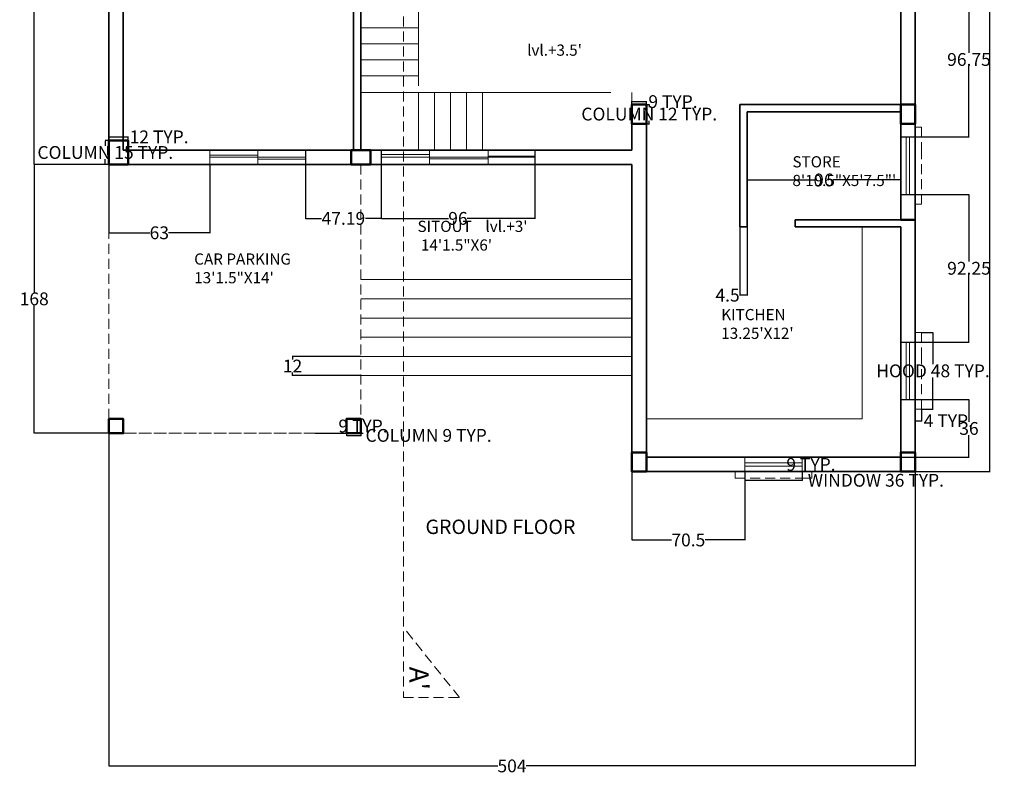
# Model space of a CAD drawing. Units: inches. Extents: x 683 to 1299, y -12 to 932.
# Tile 1 of 3: x 683 to 1299, y -12 to 460. Entities that reach past the tile are written whole.
import ezdxf

# ---------------------------------------------------------------- set-up
doc = ezdxf.new("R2010")
doc.units = ezdxf.units.IN
doc.header["$LTSCALE"] = 25
doc.header["$MEASUREMENT"] = 0
doc.linetypes.add('HIDDEN', pattern=[0.375, 0.25, -0.125])
for name, color, linetype, lineweight in [('A-ANNO-DIMS', 2, 'Continuous', 18), ('A-ANNO-SECT', 7, 'HIDDEN', 18), ('A-ANNO-SYMB', 6, 'Continuous', 18), ('A-ANNO-TEXT', 6, 'Continuous', 25), ('A-AREA-IDEN', 6, 'Continuous', 18), ('A-COLS', 1, 'Continuous', 50), ('A-FLOR', 7, 'Continuous', 25), ('A-FLOR-FIXT', 8, 'Continuous', 18), ('A-FLOR-STRS', 7, 'Continuous', 18), ('A-FLOR-STRS-HIDN', 5, 'HIDDEN', 18), ('A-GLAZ-OVHD', 7, 'HIDDEN', 13), ('A-ROOF-OVHD', 7, 'HIDDEN', 18), ('A-WALL', 7, 'Continuous', 35)]:
    doc.layers.add(name, color=color, linetype=linetype, lineweight=lineweight)
doc.layers.add('A-GLAZ', color=41, linetype='Continuous', lineweight=18, true_color=0xf4ee51)
doc.styles.get("Standard").update_dxf_attribs({"font": 'arial.ttf'})
doc.dimstyles.get("Standard").update_dxf_attribs({"dimtxt": 8, "dimasz": 0.18, "dimexe": 0.18, "dimexo": 0.0625, "dimgap": 0.09, "dimtad": 0, "dimtih": 1, "dimtoh": 1, "dimdec": 1, "dimzin": 0, "dimdsep": 46, "dimlunit": 3, "dimtxsty": 'Standard', "dimcen": 0.09, "dimadec": 0, "dimazin": 0, "dimtfac": 1, "dimtdec": 1, "dimtofl": 0, "dimtmove": 0, "dimatfit": 3, "dimfxl": 1, "dimtolj": 1, "dimtzin": 0, "dimarcsym": 0})

# ---------------------------------------------------------------- blocks, each defined once
blk = doc.blocks.new('WIN-SLIDER-60IN')
for p, q in [((60, 9), (0, 9)), ((0, 9), (0, 0)), ((30, 9), (30, 0)), ((60, 0), (60, 9)), ((0, 0), (60, 0)), ((30, 0), (60, 0))]:
    blk.add_line(p, q)
for points in [[(30, 4.5), (0, 4.5), (0, 5.76), (30, 5.76)], [(60, 3.24), (30, 3.24), (30, 4.5), (60, 4.5)]]:
    blk.add_lwpolyline(points, close=True)
blk = doc.blocks.new('WIN-36IN')
for p, q in [((36, 9), (0, 9)), ((0, 9), (0, 0)), ((36, 0), (36, 9)), ((0, 5.5), (36, 5.5)), ((0, 3.5), (36, 3.5)), ((0, 0), (36, 0))]:
    blk.add_line(p, q)
blk = doc.blocks.new('COLUMN-12X15IN')
blk.add_lwpolyline([(0, 0), (12, 0), (12, 15), (0, 15)], close=True)
blk = doc.blocks.new('COLUMN-12X9IN')
blk.add_lwpolyline([(0, 9), (0, 0), (12, 0), (12, 9)], close=True)
blk = doc.blocks.new('COLUMN-9X9IN')
blk.add_lwpolyline([(0, 0), (9, 0), (9, 9), (0, 9)], close=True)
blk = doc.blocks.new('WIN-HOOD-36IN')
for p, q in [((0, 48), (4, 48)), ((4, 48), (4, 33.44)), ((4, 0), (4, 33.44)), ((0, 0), (4, 0))]:
    blk.add_line(p, q)
blk = doc.blocks.new('*D14')
at = {"layer": 'A-ANNO-DIMS', "color": 0, "lineweight": -2, "ltscale": 25, "transparency": 16777216}
for p, q in [((1075.04, 407.1), (1076.95, 407.1)), ((1076.77, 406.92), (1076.77, 405.33)), ((1075.04, 395.1), (1076.95, 395.1)), ((1076.77, 395.28), (1076.77, 396.87))]:
    blk.add_line(p, q, dxfattribs=at)
at = {"layer": 'A-ANNO-DIMS', "color": 0, "ltscale": 25, "transparency": 16777216}
for points in [[(1076.74, 406.92), (1076.8, 406.92), (1076.77, 407.1)], [(1076.74, 395.28), (1076.8, 395.28), (1076.77, 395.1)]]:
    blk.add_solid(points, dxfattribs=at)
at = {"layer": 'Defpoints', "color": 0, "ltscale": 25, "transparency": 16777216}
for p in [(1074.97, 407.1), (1074.97, 395.1), (1076.77, 395.1)]:
    blk.add_point(p, dxfattribs=at)
at = {"layer": 'A-ANNO-DIMS', "color": 0, "ltscale": 25, "transparency": 16777216, "insert": (1076.77, 401.1), "char_height": 8, "attachment_point": 5}
blk.add_mtext('\\A1;COLUMN 12 TYP.', dxfattribs=at)
blk = doc.blocks.new('*D15')
at = {"layer": 'A-ANNO-DIMS', "color": 0, "lineweight": -2, "ltscale": 25, "transparency": 16777216}
for p, q in [((1065.97, 407.16), (1065.97, 409.08)), ((1066.15, 408.9), (1074.79, 408.9)), ((1074.97, 407.16), (1074.97, 409.08)), ((1074.97, 408.9), (1075.15, 408.9))]:
    blk.add_line(p, q, dxfattribs=at)
at = {"layer": 'A-ANNO-DIMS', "color": 0, "ltscale": 25, "transparency": 16777216}
for points in [[(1066.15, 408.93), (1066.15, 408.87), (1065.97, 408.9)], [(1074.79, 408.93), (1074.79, 408.87), (1074.97, 408.9)]]:
    blk.add_solid(points, dxfattribs=at)
at = {"layer": 'Defpoints', "color": 0, "ltscale": 25, "transparency": 16777216}
for p in [(1065.97, 407.1), (1074.97, 408.9), (1074.97, 407.1)]:
    blk.add_point(p, dxfattribs=at)
at = {"layer": 'A-ANNO-DIMS', "color": 0, "ltscale": 25, "transparency": 16777216, "insert": (1091.61, 408.9), "char_height": 8, "attachment_point": 5}
blk.add_mtext('\\A1;9 TYP.', dxfattribs=at)
blk = doc.blocks.new('*D16')
at = {"layer": 'A-ANNO-DIMS', "color": 0, "lineweight": -2, "ltscale": 25, "transparency": 16777216}
for p, q in [((1136.47, 177.54), (1136.47, 172.02)), ((1172.47, 177.54), (1172.47, 172.02)), ((1136.65, 172.2), (1172.29, 172.2)), ((1172.47, 172.2), (1172.65, 172.2))]:
    blk.add_line(p, q, dxfattribs=at)
at = {"layer": 'A-ANNO-DIMS', "color": 0, "ltscale": 25, "transparency": 16777216}
for points in [[(1136.65, 172.23), (1136.65, 172.17), (1136.47, 172.2)], [(1172.29, 172.23), (1172.29, 172.17), (1172.47, 172.2)]]:
    blk.add_solid(points, dxfattribs=at)
at = {"layer": 'Defpoints', "color": 0, "ltscale": 25, "transparency": 16777216}
for p in [(1136.47, 177.6), (1172.47, 177.6), (1172.47, 172.2)]:
    blk.add_point(p, dxfattribs=at)
at = {"layer": 'A-ANNO-DIMS', "color": 0, "ltscale": 25, "transparency": 16777216, "insert": (1218.45, 172.2), "char_height": 8, "attachment_point": 5}
blk.add_mtext('\\A1;WINDOW 36 TYP.', dxfattribs=at)
blk = doc.blocks.new('*D17')
at = {"layer": 'A-ANNO-DIMS', "color": 0, "lineweight": -2, "ltscale": 25, "transparency": 16777216}
for p, q in [((1172.54, 186.6), (1178.05, 186.6)), ((1177.87, 186.42), (1177.87, 186.27)), ((1172.54, 177.6), (1178.05, 177.6)), ((1177.87, 177.78), (1177.87, 177.92))]:
    blk.add_line(p, q, dxfattribs=at)
at = {"layer": 'A-ANNO-DIMS', "color": 0, "ltscale": 25, "transparency": 16777216}
for points in [[(1177.84, 186.42), (1177.9, 186.42), (1177.87, 186.6)], [(1177.84, 177.78), (1177.9, 177.78), (1177.87, 177.6)]]:
    blk.add_solid(points, dxfattribs=at)
at = {"layer": 'Defpoints', "color": 0, "ltscale": 25, "transparency": 16777216}
for p in [(1172.47, 186.6), (1177.87, 186.6), (1172.47, 177.6)]:
    blk.add_point(p, dxfattribs=at)
at = {"layer": 'A-ANNO-DIMS', "color": 0, "ltscale": 25, "transparency": 16777216, "insert": (1177.87, 182.1), "char_height": 8, "attachment_point": 5}
blk.add_mtext('\\A1;9 TYP.', dxfattribs=at)
blk = doc.blocks.new('*D20')
at = {"layer": 'A-ANNO-DIMS', "color": 0, "lineweight": -2, "ltscale": 25, "transparency": 16777216}
for p, q in [((738.91, 384.6), (736.54, 384.6)), ((736.72, 384.42), (736.72, 381.33)), ((738.91, 369.6), (736.54, 369.6)), ((736.72, 369.78), (736.72, 372.87))]:
    blk.add_line(p, q, dxfattribs=at)
at = {"layer": 'A-ANNO-DIMS', "color": 0, "ltscale": 25, "transparency": 16777216}
for points in [[(736.69, 384.42), (736.75, 384.42), (736.72, 384.6)], [(736.69, 369.78), (736.75, 369.78), (736.72, 369.6)]]:
    blk.add_solid(points, dxfattribs=at)
at = {"layer": 'Defpoints', "color": 0, "ltscale": 25, "transparency": 16777216}
for p in [(736.72, 384.6), (738.97, 384.6), (738.97, 369.6)]:
    blk.add_point(p, dxfattribs=at)
at = {"layer": 'A-ANNO-DIMS', "color": 0, "ltscale": 25, "transparency": 16777216, "insert": (736.72, 377.1), "char_height": 8, "attachment_point": 5}
blk.add_mtext('\\A1;COLUMN 15 TYP.', dxfattribs=at)
blk = doc.blocks.new('*D21')
at = {"layer": 'A-ANNO-DIMS', "color": 0, "lineweight": -2, "ltscale": 25, "transparency": 16777216}
for p, q in [((738.97, 384.66), (738.97, 387.03)), ((739.15, 386.85), (750.79, 386.85)), ((750.97, 384.66), (750.97, 387.03)), ((750.97, 386.85), (751.15, 386.85))]:
    blk.add_line(p, q, dxfattribs=at)
at = {"layer": 'A-ANNO-DIMS', "color": 0, "ltscale": 25, "transparency": 16777216}
for points in [[(739.15, 386.88), (739.15, 386.82), (738.97, 386.85)], [(750.79, 386.88), (750.79, 386.82), (750.97, 386.85)]]:
    blk.add_solid(points, dxfattribs=at)
at = {"layer": 'Defpoints', "color": 0, "ltscale": 25, "transparency": 16777216}
for p in [(738.97, 384.6), (750.97, 386.85), (750.97, 384.6)]:
    blk.add_point(p, dxfattribs=at)
at = {"layer": 'A-ANNO-DIMS', "color": 0, "ltscale": 25, "transparency": 16777216, "insert": (770.34, 386.85), "char_height": 8, "attachment_point": 5}
blk.add_mtext('\\A1;12 TYP.', dxfattribs=at)
blk = doc.blocks.new('*D22')
at = {"layer": 'A-ANNO-DIMS', "color": 0, "lineweight": -2, "ltscale": 25, "transparency": 16777216}
for p, q in [((887.47, 201.54), (887.47, 200.07)), ((887.65, 200.25), (896.29, 200.25)), ((896.47, 201.54), (896.47, 200.07)), ((896.47, 200.25), (896.65, 200.25))]:
    blk.add_line(p, q, dxfattribs=at)
at = {"layer": 'A-ANNO-DIMS', "color": 0, "ltscale": 25, "transparency": 16777216}
for points in [[(887.65, 200.28), (887.65, 200.22), (887.47, 200.25)], [(896.29, 200.28), (896.29, 200.22), (896.47, 200.25)]]:
    blk.add_solid(points, dxfattribs=at)
at = {"layer": 'Defpoints', "color": 0, "ltscale": 25, "transparency": 16777216}
for p in [(887.47, 201.6), (896.47, 201.6), (896.47, 200.25)]:
    blk.add_point(p, dxfattribs=at)
at = {"layer": 'A-ANNO-DIMS', "color": 0, "ltscale": 25, "transparency": 16777216, "insert": (938.83, 200.25), "char_height": 8, "attachment_point": 5}
blk.add_mtext('\\A1;COLUMN 9 TYP.', dxfattribs=at)
blk = doc.blocks.new('*D23')
at = {"layer": 'A-ANNO-DIMS', "color": 0, "lineweight": -2, "ltscale": 25, "transparency": 16777216}
for p, q in [((896.54, 210.6), (898, 210.6)), ((897.82, 210.42), (897.82, 210.27)), ((896.54, 201.6), (898, 201.6)), ((897.82, 201.78), (897.82, 201.92))]:
    blk.add_line(p, q, dxfattribs=at)
at = {"layer": 'A-ANNO-DIMS', "color": 0, "ltscale": 25, "transparency": 16777216}
for points in [[(897.79, 210.42), (897.85, 210.42), (897.82, 210.6)], [(897.79, 201.78), (897.85, 201.78), (897.82, 201.6)]]:
    blk.add_solid(points, dxfattribs=at)
at = {"layer": 'Defpoints', "color": 0, "ltscale": 25, "transparency": 16777216}
for p in [(896.47, 210.6), (897.82, 210.6), (896.47, 201.6)]:
    blk.add_point(p, dxfattribs=at)
at = {"layer": 'A-ANNO-DIMS', "color": 0, "ltscale": 25, "transparency": 16777216, "insert": (897.82, 206.1), "char_height": 8, "attachment_point": 5}
blk.add_mtext('\\A1;9 TYP.', dxfattribs=at)
blk = doc.blocks.new('*D28')
at = {"layer": 'A-ANNO-DIMS', "color": 0, "lineweight": -2, "ltscale": 25, "transparency": 16777216}
for p, q in [((1247.04, 264.6), (1254.35, 264.6)), ((1254.17, 264.42), (1254.17, 244.83)), ((1254.17, 216.78), (1254.17, 236.37)), ((1247.04, 216.6), (1254.35, 216.6))]:
    blk.add_line(p, q, dxfattribs=at)
at = {"layer": 'A-ANNO-DIMS', "color": 0, "ltscale": 25, "transparency": 16777216}
for points in [[(1254.14, 264.42), (1254.2, 264.42), (1254.17, 264.6)], [(1254.14, 216.78), (1254.2, 216.78), (1254.17, 216.6)]]:
    blk.add_solid(points, dxfattribs=at)
at = {"layer": 'Defpoints', "color": 0, "ltscale": 25, "transparency": 16777216}
for p in [(1246.97, 264.6), (1254.17, 264.6), (1246.97, 216.6)]:
    blk.add_point(p, dxfattribs=at)
at = {"layer": 'A-ANNO-DIMS', "color": 0, "ltscale": 25, "transparency": 16777216, "insert": (1254.17, 240.6), "char_height": 8, "attachment_point": 5}
blk.add_mtext('\\A1;HOOD 48 TYP.', dxfattribs=at)
blk = doc.blocks.new('*D29')
at = {"layer": 'A-ANNO-DIMS', "color": 0, "lineweight": -2, "ltscale": 25, "transparency": 16777216}
for p, q in [((1242.97, 216.54), (1242.97, 209.22)), ((1246.97, 216.54), (1246.97, 209.22)), ((1243.15, 209.4), (1246.79, 209.4)), ((1246.97, 209.4), (1247.15, 209.4))]:
    blk.add_line(p, q, dxfattribs=at)
at = {"layer": 'A-ANNO-DIMS', "color": 0, "ltscale": 25, "transparency": 16777216}
for points in [[(1243.15, 209.43), (1243.15, 209.37), (1242.97, 209.4)], [(1246.79, 209.43), (1246.79, 209.37), (1246.97, 209.4)]]:
    blk.add_solid(points, dxfattribs=at)
at = {"layer": 'Defpoints', "color": 0, "ltscale": 25, "transparency": 16777216}
for p in [(1242.97, 216.6), (1246.97, 216.6), (1246.97, 209.4)]:
    blk.add_point(p, dxfattribs=at)
at = {"layer": 'A-ANNO-DIMS', "color": 0, "ltscale": 25, "transparency": 16777216, "insert": (1263.77, 209.4), "char_height": 8, "attachment_point": 5}
blk.add_mtext('\\A1;4 TYP.', dxfattribs=at)
blk = doc.blocks.new('*D32')
at = {"layer": 'A-ANNO-DIMS', "color": 0, "lineweight": -2, "ltscale": 25, "transparency": 16777216}
for p, q in [((738.97, 201.54), (738.97, -6.53)), ((1242.97, 177.54), (1242.97, -6.53)), ((739.15, -6.35), (982.06, -6.35)), ((1242.79, -6.35), (999.88, -6.35))]:
    blk.add_line(p, q, dxfattribs=at)
at = {"layer": 'A-ANNO-DIMS', "color": 0, "ltscale": 25, "transparency": 16777216}
for points in [[(739.15, -6.32), (739.15, -6.38), (738.97, -6.35)], [(1242.79, -6.32), (1242.79, -6.38), (1242.97, -6.35)]]:
    blk.add_solid(points, dxfattribs=at)
at = {"layer": 'Defpoints', "color": 0, "ltscale": 25, "transparency": 16777216}
for p in [(738.97, 201.6), (1242.97, 177.6), (1242.97, -6.35)]:
    blk.add_point(p, dxfattribs=at)
at = {"layer": 'A-ANNO-DIMS', "color": 0, "ltscale": 25, "transparency": 16777216, "insert": (990.97, -6.35), "char_height": 8, "attachment_point": 5}
blk.add_mtext('\\A1;504', dxfattribs=at)
blk = doc.blocks.new('*D33')
at = {"layer": 'A-ANNO-DIMS', "color": 0, "lineweight": -2, "ltscale": 25, "transparency": 16777216}
for p, q in [((1243.04, 825.6), (1289.85, 825.6)), ((1289.67, 825.42), (1289.67, 505.77)), ((1289.67, 177.78), (1289.67, 497.42)), ((1243.04, 177.6), (1289.85, 177.6))]:
    blk.add_line(p, q, dxfattribs=at)
at = {"layer": 'A-ANNO-DIMS', "color": 0, "ltscale": 25, "transparency": 16777216}
for points in [[(1289.64, 825.42), (1289.7, 825.42), (1289.67, 825.6)], [(1289.64, 177.78), (1289.7, 177.78), (1289.67, 177.6)]]:
    blk.add_solid(points, dxfattribs=at)
at = {"layer": 'Defpoints', "color": 0, "ltscale": 25, "transparency": 16777216}
for p in [(1242.97, 825.6), (1289.67, 825.6), (1242.97, 177.6)]:
    blk.add_point(p, dxfattribs=at)
at = {"layer": 'A-ANNO-DIMS', "color": 0, "ltscale": 25, "transparency": 16777216, "insert": (1289.67, 501.6), "char_height": 8, "attachment_point": 5}
blk.add_mtext('\\A1;648', dxfattribs=at)
blk = doc.blocks.new('*D40')
at = {"layer": 'A-ANNO-DIMS', "color": 0, "lineweight": -2, "ltscale": 25, "transparency": 16777216}
for p, q in [((738.91, 369.6), (692.09, 369.6)), ((692.27, 369.42), (692.27, 289.77)), ((692.27, 201.78), (692.27, 281.42)), ((738.91, 201.6), (692.09, 201.6))]:
    blk.add_line(p, q, dxfattribs=at)
at = {"layer": 'A-ANNO-DIMS', "color": 0, "ltscale": 25, "transparency": 16777216}
for points in [[(692.24, 369.42), (692.3, 369.42), (692.27, 369.6)], [(692.24, 201.78), (692.3, 201.78), (692.27, 201.6)]]:
    blk.add_solid(points, dxfattribs=at)
at = {"layer": 'Defpoints', "color": 0, "ltscale": 25, "transparency": 16777216}
for p in [(692.27, 369.6), (738.97, 369.6), (738.97, 201.6)]:
    blk.add_point(p, dxfattribs=at)
at = {"layer": 'A-ANNO-DIMS', "color": 0, "ltscale": 25, "transparency": 16777216, "insert": (692.27, 285.6), "char_height": 8, "attachment_point": 5}
blk.add_mtext('\\A1;168', dxfattribs=at)
blk = doc.blocks.new('*D41')
at = {"layer": 'A-ANNO-DIMS', "color": 0, "lineweight": -2, "ltscale": 25, "transparency": 16777216}
for p, q in [((738.91, 570.6), (692.09, 570.6)), ((692.27, 570.42), (692.27, 474.27)), ((692.27, 369.78), (692.27, 465.92)), ((738.91, 369.6), (692.09, 369.6))]:
    blk.add_line(p, q, dxfattribs=at)
at = {"layer": 'A-ANNO-DIMS', "color": 0, "ltscale": 25, "transparency": 16777216}
for points in [[(692.24, 570.42), (692.3, 570.42), (692.27, 570.6)], [(692.24, 369.78), (692.3, 369.78), (692.27, 369.6)]]:
    blk.add_solid(points, dxfattribs=at)
at = {"layer": 'Defpoints', "color": 0, "ltscale": 25, "transparency": 16777216}
for p in [(692.27, 570.6), (738.97, 570.6), (738.97, 369.6)]:
    blk.add_point(p, dxfattribs=at)
at = {"layer": 'A-ANNO-DIMS', "color": 0, "ltscale": 25, "transparency": 16777216, "insert": (692.27, 470.1), "char_height": 8, "attachment_point": 5}
blk.add_mtext('\\A1;201', dxfattribs=at)
blk = doc.blocks.new('*D47')
at = {"layer": 'A-ANNO-DIMS', "color": 0, "lineweight": -2, "ltscale": 25, "transparency": 16777216}
for p, q in [((1234.04, 483.6), (1276.85, 483.6)), ((1276.67, 483.42), (1276.67, 439.4)), ((1276.67, 387.03), (1276.67, 431.05)), ((1234.04, 386.85), (1276.85, 386.85))]:
    blk.add_line(p, q, dxfattribs=at)
at = {"layer": 'A-ANNO-DIMS', "color": 0, "ltscale": 25, "transparency": 16777216}
for points in [[(1276.64, 483.42), (1276.7, 483.42), (1276.67, 483.6)], [(1276.64, 387.03), (1276.7, 387.03), (1276.67, 386.85)]]:
    blk.add_solid(points, dxfattribs=at)
at = {"layer": 'Defpoints', "color": 0, "ltscale": 25, "transparency": 16777216}
for p in [(1233.97, 483.6), (1233.97, 386.85), (1276.67, 386.85)]:
    blk.add_point(p, dxfattribs=at)
at = {"layer": 'A-ANNO-DIMS', "color": 0, "ltscale": 25, "transparency": 16777216, "insert": (1276.67, 435.22), "char_height": 8, "attachment_point": 5}
blk.add_mtext('\\A1;96.75', dxfattribs=at)
blk = doc.blocks.new('*D48')
at = {"layer": 'A-ANNO-DIMS', "color": 0, "lineweight": -2, "ltscale": 25, "transparency": 16777216}
for p, q in [((1234.04, 350.85), (1276.85, 350.85)), ((1276.67, 350.67), (1276.67, 308.9)), ((1276.67, 258.78), (1276.67, 300.55)), ((1234.04, 258.6), (1276.85, 258.6))]:
    blk.add_line(p, q, dxfattribs=at)
at = {"layer": 'A-ANNO-DIMS', "color": 0, "ltscale": 25, "transparency": 16777216}
for points in [[(1276.64, 350.67), (1276.7, 350.67), (1276.67, 350.85)], [(1276.64, 258.78), (1276.7, 258.78), (1276.67, 258.6)]]:
    blk.add_solid(points, dxfattribs=at)
at = {"layer": 'Defpoints', "color": 0, "ltscale": 25, "transparency": 16777216}
for p in [(1233.97, 350.85), (1233.97, 258.6), (1276.67, 258.6)]:
    blk.add_point(p, dxfattribs=at)
at = {"layer": 'A-ANNO-DIMS', "color": 0, "ltscale": 25, "transparency": 16777216, "insert": (1276.67, 304.72), "char_height": 8, "attachment_point": 5}
blk.add_mtext('\\A1;92.25', dxfattribs=at)
blk = doc.blocks.new('*D49')
at = {"layer": 'A-ANNO-DIMS', "color": 0, "lineweight": -2, "ltscale": 25, "transparency": 16777216}
for p, q in [((1234.04, 222.6), (1276.85, 222.6)), ((1276.67, 222.42), (1276.67, 208.78)), ((1276.67, 186.78), (1276.67, 200.42)), ((1234.04, 186.6), (1276.85, 186.6))]:
    blk.add_line(p, q, dxfattribs=at)
at = {"layer": 'A-ANNO-DIMS', "color": 0, "ltscale": 25, "transparency": 16777216}
for points in [[(1276.64, 222.42), (1276.7, 222.42), (1276.67, 222.6)], [(1276.64, 186.78), (1276.7, 186.78), (1276.67, 186.6)]]:
    blk.add_solid(points, dxfattribs=at)
at = {"layer": 'Defpoints', "color": 0, "ltscale": 25, "transparency": 16777216}
for p in [(1233.97, 222.6), (1233.97, 186.6), (1276.67, 186.6)]:
    blk.add_point(p, dxfattribs=at)
at = {"layer": 'A-ANNO-DIMS', "color": 0, "ltscale": 25, "transparency": 16777216, "insert": (1276.67, 204.6), "char_height": 8, "attachment_point": 5}
blk.add_mtext('\\A1;36', dxfattribs=at)
blk = doc.blocks.new('*D52')
at = {"layer": 'A-ANNO-DIMS', "color": 0, "lineweight": -2, "ltscale": 25, "transparency": 16777216}
for p, q in [((896.41, 249.6), (853.59, 249.6)), ((853.77, 249.42), (853.77, 247.71)), ((896.41, 237.6), (853.59, 237.6)), ((853.77, 237.78), (853.77, 239.49))]:
    blk.add_line(p, q, dxfattribs=at)
at = {"layer": 'A-ANNO-DIMS', "color": 0, "ltscale": 25, "transparency": 16777216}
for points in [[(853.74, 249.42), (853.8, 249.42), (853.77, 249.6)], [(853.74, 237.78), (853.8, 237.78), (853.77, 237.6)]]:
    blk.add_solid(points, dxfattribs=at)
at = {"layer": 'Defpoints', "color": 0, "ltscale": 25, "transparency": 16777216}
for p in [(853.77, 249.6), (896.47, 249.6), (896.47, 237.6)]:
    blk.add_point(p, dxfattribs=at)
at = {"layer": 'A-ANNO-DIMS', "color": 0, "ltscale": 25, "transparency": 16777216, "insert": (853.77, 243.6), "char_height": 8, "attachment_point": 5}
blk.add_mtext('\\A1;12', dxfattribs=at)
blk = doc.blocks.new('*D55')
at = {"layer": 'A-ANNO-DIMS', "color": 0, "lineweight": -2, "ltscale": 25, "transparency": 16777216}
for p, q in [((738.97, 369.54), (738.97, 326.72)), ((801.97, 369.54), (801.97, 326.72)), ((739.15, 326.9), (764.63, 326.9)), ((801.79, 326.9), (776.31, 326.9))]:
    blk.add_line(p, q, dxfattribs=at)
at = {"layer": 'A-ANNO-DIMS', "color": 0, "ltscale": 25, "transparency": 16777216}
for points in [[(739.15, 326.93), (739.15, 326.87), (738.97, 326.9)], [(801.79, 326.93), (801.79, 326.87), (801.97, 326.9)]]:
    blk.add_solid(points, dxfattribs=at)
at = {"layer": 'Defpoints', "color": 0, "ltscale": 25, "transparency": 16777216}
for p in [(738.97, 369.6), (801.97, 369.6), (738.97, 326.9)]:
    blk.add_point(p, dxfattribs=at)
at = {"layer": 'A-ANNO-DIMS', "color": 0, "ltscale": 25, "transparency": 16777216, "insert": (770.47, 326.9), "char_height": 8, "attachment_point": 5}
blk.add_mtext('\\A1;63', dxfattribs=at)
blk = doc.blocks.new('*D56')
at = {"layer": 'A-ANNO-DIMS', "color": 0, "lineweight": -2, "ltscale": 25, "transparency": 16777216}
for p, q in [((861.97, 378.54), (861.97, 335.72)), ((909.17, 378.54), (909.17, 335.72)), ((862.15, 335.9), (871.81, 335.9)), ((908.99, 335.9), (899.33, 335.9))]:
    blk.add_line(p, q, dxfattribs=at)
at = {"layer": 'A-ANNO-DIMS', "color": 0, "ltscale": 25, "transparency": 16777216}
for points in [[(862.15, 335.93), (862.15, 335.87), (861.97, 335.9)], [(908.99, 335.93), (908.99, 335.87), (909.17, 335.9)]]:
    blk.add_solid(points, dxfattribs=at)
at = {"layer": 'Defpoints', "color": 0, "ltscale": 25, "transparency": 16777216}
for p in [(861.97, 378.6), (909.17, 378.6), (861.97, 335.9)]:
    blk.add_point(p, dxfattribs=at)
at = {"layer": 'A-ANNO-DIMS', "color": 0, "ltscale": 25, "transparency": 16777216, "insert": (885.57, 335.9), "char_height": 8, "attachment_point": 5}
blk.add_mtext('\\A1;47.19', dxfattribs=at)
blk = doc.blocks.new('*D57')
at = {"layer": 'A-ANNO-DIMS', "color": 0, "lineweight": -2, "ltscale": 25, "transparency": 16777216}
for p, q in [((909.17, 378.54), (909.17, 335.72)), ((1005.17, 378.54), (1005.17, 335.72)), ((909.35, 335.9), (951.35, 335.9)), ((1004.99, 335.9), (962.98, 335.9))]:
    blk.add_line(p, q, dxfattribs=at)
at = {"layer": 'A-ANNO-DIMS', "color": 0, "ltscale": 25, "transparency": 16777216}
for points in [[(909.35, 335.93), (909.35, 335.87), (909.17, 335.9)], [(1004.99, 335.93), (1004.99, 335.87), (1005.17, 335.9)]]:
    blk.add_solid(points, dxfattribs=at)
at = {"layer": 'Defpoints', "color": 0, "ltscale": 25, "transparency": 16777216}
for p in [(909.17, 378.6), (1005.17, 378.6), (909.17, 335.9)]:
    blk.add_point(p, dxfattribs=at)
at = {"layer": 'A-ANNO-DIMS', "color": 0, "ltscale": 25, "transparency": 16777216, "insert": (957.17, 335.9), "char_height": 8, "attachment_point": 5}
blk.add_mtext('\\A1;96', dxfattribs=at)
blk = doc.blocks.new('*D58')
at = {"layer": 'A-ANNO-DIMS', "color": 0, "lineweight": -2, "ltscale": 25, "transparency": 16777216}
for p, q in [((1065.97, 177.54), (1065.97, 134.72)), ((1136.47, 177.54), (1136.47, 134.72)), ((1066.15, 134.9), (1090.75, 134.9)), ((1136.29, 134.9), (1111.7, 134.9))]:
    blk.add_line(p, q, dxfattribs=at)
at = {"layer": 'A-ANNO-DIMS', "color": 0, "ltscale": 25, "transparency": 16777216}
for points in [[(1066.15, 134.93), (1066.15, 134.87), (1065.97, 134.9)], [(1136.29, 134.93), (1136.29, 134.87), (1136.47, 134.9)]]:
    blk.add_solid(points, dxfattribs=at)
at = {"layer": 'Defpoints', "color": 0, "ltscale": 25, "transparency": 16777216}
for p in [(1065.97, 177.6), (1136.47, 177.6), (1065.97, 134.9)]:
    blk.add_point(p, dxfattribs=at)
at = {"layer": 'A-ANNO-DIMS', "color": 0, "ltscale": 25, "transparency": 16777216, "insert": (1101.22, 134.9), "char_height": 8, "attachment_point": 5}
blk.add_mtext('\\A1;70.5', dxfattribs=at)
blk = doc.blocks.new('*D59')
at = {"layer": 'A-ANNO-DIMS', "color": 0, "lineweight": -2, "ltscale": 25, "transparency": 16777216}
for p, q in [((1137.97, 402.54), (1137.97, 359.72)), ((1233.97, 402.54), (1233.97, 359.72)), ((1138.15, 359.9), (1180.16, 359.9)), ((1233.79, 359.9), (1191.79, 359.9))]:
    blk.add_line(p, q, dxfattribs=at)
at = {"layer": 'A-ANNO-DIMS', "color": 0, "ltscale": 25, "transparency": 16777216}
for points in [[(1138.15, 359.93), (1138.15, 359.87), (1137.97, 359.9)], [(1233.79, 359.93), (1233.79, 359.87), (1233.97, 359.9)]]:
    blk.add_solid(points, dxfattribs=at)
at = {"layer": 'Defpoints', "color": 0, "ltscale": 25, "transparency": 16777216}
for p in [(1137.97, 402.6), (1233.97, 402.6), (1137.97, 359.9)]:
    blk.add_point(p, dxfattribs=at)
at = {"layer": 'A-ANNO-DIMS', "color": 0, "ltscale": 25, "transparency": 16777216, "insert": (1185.97, 359.9), "char_height": 8, "attachment_point": 5}
blk.add_mtext('\\A1;96', dxfattribs=at)
blk = doc.blocks.new('*D60')
at = {"layer": 'A-ANNO-DIMS', "color": 0, "lineweight": -2, "ltscale": 25, "transparency": 16777216}
for p, q in [((1133.47, 330.54), (1133.47, 287.72)), ((1137.97, 330.54), (1137.97, 287.72)), ((1133.47, 287.9), (1133.29, 287.9)), ((1137.79, 287.9), (1133.65, 287.9))]:
    blk.add_line(p, q, dxfattribs=at)
at = {"layer": 'A-ANNO-DIMS', "color": 0, "ltscale": 25, "transparency": 16777216}
for points in [[(1133.65, 287.93), (1133.65, 287.87), (1133.47, 287.9)], [(1137.79, 287.93), (1137.79, 287.87), (1137.97, 287.9)]]:
    blk.add_solid(points, dxfattribs=at)
at = {"layer": 'Defpoints', "color": 0, "ltscale": 25, "transparency": 16777216}
for p in [(1133.47, 330.6), (1137.97, 330.6), (1133.47, 287.9)]:
    blk.add_point(p, dxfattribs=at)
at = {"layer": 'A-ANNO-DIMS', "color": 0, "ltscale": 25, "transparency": 16777216, "insert": (1125.73, 287.9), "char_height": 8, "attachment_point": 5}
blk.add_mtext('\\A1;4.5', dxfattribs=at)

msp = doc.modelspace()

# ---------------------------------------------------------------- linework, layer by layer
at = {"layer": 'A-ANNO-SECT'}
for p, q in [((923.068, 883.972), (923.068, 36.355)), ((958.231, 36.355), (923.068, 80.211)), ((923.068, 36.355), (958.231, 36.355))]:
    msp.add_line(p, q, dxfattribs=at)
at = {"layer": 'A-COLS'}
for p, q in [((1065.973, 407.099), (1074.973, 407.099)), ((1233.973, 407.099), (1242.973, 407.099)), ((1233.973, 335.099), (1242.973, 335.099)), ((738.973, 210.599), (738.973, 201.599)), ((1065.973, 189.599), (1074.973, 189.599)), ((1233.973, 189.599), (1242.973, 189.599))]:
    msp.add_line(p, q, dxfattribs=at)
at = {"layer": 'A-FLOR'}
for p, q in [((896.473, 369.599), (1065.973, 369.599)), ((867.973, 201.599), (896.473, 201.599))]:
    msp.add_line(p, q, dxfattribs=at)
at = {"layer": 'A-FLOR-FIXT'}
for p in [(1209.973, 330.599), (1074.973, 210.599)]:
    msp.add_line(p, (1209.973, 210.599), dxfattribs=at)
at = {"layer": 'A-FLOR-STRS'}
for p, q in [((896.473, 297.599), (1065.973, 297.599)), ((896.473, 285.599), (1065.973, 285.599)), ((896.473, 273.599), (1065.973, 273.599)), ((896.473, 261.599), (1065.973, 261.599)), ((896.473, 249.599), (1065.973, 249.599)), ((896.473, 237.599), (1065.973, 237.599))]:
    msp.add_line(p, q, dxfattribs=at)
at = {"layer": 'A-FLOR-STRS-HIDN', "ltscale": 25}
for p, q in [((932.473, 575.099), (932.473, 378.599)), ((932.473, 455.099), (896.473, 455.099)), ((932.473, 445.099), (896.473, 445.099)), ((932.473, 435.099), (896.473, 435.099)), ((932.473, 425.099), (896.473, 425.099)), ((896.473, 414.599), (1065.973, 414.599)), ((932.473, 414.618), (898.973, 414.618)), ((932.473, 414.618), (898.973, 414.618)), ((932.473, 414.618), (898.973, 414.618)), ((932.473, 414.599), (932.473, 378.599)), ((942.473, 414.599), (942.473, 378.599)), ((952.473, 414.599), (952.473, 378.599)), ((962.473, 414.599), (962.473, 378.599)), ((972.473, 414.599), (972.473, 378.599)), ((1065.973, 407.099), (1065.973, 414.599))]:
    msp.add_line(p, q, dxfattribs=at)
at = {"layer": 'A-GLAZ'}
for p, q in [((1242.973, 386.849), (1242.973, 392.849)), ((1233.973, 368.849), (1233.973, 386.849)), ((1242.973, 350.849), (1242.973, 386.849)), ((801.973, 369.599), (801.973, 378.599)), ((801.973, 378.599), (837.973, 378.599)), ((819.973, 378.599), (837.973, 378.599)), ((1005.166, 378.599), (909.166, 378.599)), ((909.166, 378.599), (909.166, 369.599)), ((939.348, 369.599), (939.348, 378.599)), ((975.997, 369.599), (975.997, 378.599)), ((1005.166, 369.599), (1005.166, 378.599)), ((837.973, 369.599), (801.973, 369.599)), ((909.166, 369.599), (1005.166, 369.599)), ((957.166, 369.599), (1005.166, 369.599)), ((1242.973, 350.849), (1242.973, 344.849)), ((1242.973, 258.599), (1242.973, 264.599)), ((1242.973, 222.599), (1242.973, 216.599)), ((1136.473, 177.599), (1130.473, 177.599)), ((1154.473, 177.599), (1172.473, 177.599)), ((1172.473, 177.599), (1178.473, 177.599))]:
    msp.add_line(p, q, dxfattribs=at)
for points in [[(939.348, 374.099), (909.166, 374.099), (909.166, 375.825), (939.348, 375.825)], [(939.348, 374.099), (975.997, 374.099), (975.997, 373.034), (939.348, 373.034)], [(975.997, 374.099), (1005.166, 374.099), (1005.166, 374.891), (975.997, 374.891)]]:
    msp.add_lwpolyline(points, close=True, dxfattribs=at)
at = {"layer": 'A-GLAZ-OVHD'}
for p, q in [((1130.473, 177.599), (1130.473, 173.599)), ((1130.473, 173.599), (1174.082, 173.599)), ((1178.473, 173.599), (1174.082, 173.599)), ((1178.473, 177.599), (1178.473, 173.599))]:
    msp.add_line(p, q, dxfattribs=at)
at = {"layer": 'A-ROOF-OVHD'}
for p, q in [((738.973, 210.599), (738.973, 369.599)), ((896.473, 369.599), (896.473, 201.599)), ((896.473, 369.599), (896.473, 210.599)), ((738.973, 201.599), (867.973, 201.599)), ((887.473, 201.599), (747.973, 201.599))]:
    msp.add_line(p, q, dxfattribs=at)
at = {"layer": 'A-WALL'}
for p, q in [((738.973, 825.599), (738.973, 369.599)), ((1242.973, 729.599), (1242.973, 177.599)), ((1233.973, 620.099), (1233.973, 407.099)), ((896.473, 575.099), (896.473, 378.599)), ((747.973, 570.599), (747.973, 378.599)), ((891.973, 570.599), (891.973, 378.599)), ((1065.973, 407.099), (1065.973, 378.599)), ((1074.973, 407.099), (1074.973, 251.778)), ((1133.473, 407.099), (1133.473, 330.599)), ((1133.473, 407.099), (1233.973, 407.099)), ((1137.973, 402.599), (1137.973, 335.099)), ((1137.973, 402.599), (1233.973, 402.599)), ((1233.973, 402.599), (1233.973, 335.099)), ((747.973, 378.599), (891.973, 378.599)), ((896.473, 378.599), (1065.973, 378.599)), ((738.973, 369.599), (1065.973, 369.599)), ((1065.973, 369.599), (1065.973, 177.599)), ((1137.973, 335.099), (1137.973, 330.599)), ((1167.973, 335.099), (1233.973, 335.099)), ((1167.973, 335.099), (1167.973, 330.599)), ((1074.973, 330.599), (1074.973, 186.599)), ((1133.473, 330.599), (1137.973, 330.599)), ((1167.973, 330.599), (1233.973, 330.599)), ((1233.973, 330.599), (1233.973, 186.599)), ((1074.973, 186.599), (1233.973, 186.599)), ((1065.973, 177.599), (1242.973, 177.599))]:
    msp.add_line(p, q, dxfattribs=at)

# ---------------------------------------------------------------- block references
at = {"layer": 'A-COLS'}
for p, rotation in [((1065.973, 407.099), 269.9999999999999), ((1233.973, 407.099), 269.9999999999999), ((1065.973, 189.599), 270), ((1233.973, 189.599), 270)]:
    msp.add_blockref('COLUMN-12X9IN', p, dxfattribs=dict(at, rotation=rotation))
for name, p in [('COLUMN-12X15IN', (738.973, 369.599)), ('COLUMN-12X9IN', (890.473, 369.599)), ('COLUMN-9X9IN', (738.973, 201.599)), ('COLUMN-9X9IN', (887.473, 201.599))]:
    msp.add_blockref(name, p, dxfattribs=at)
at = {"layer": 'A-GLAZ'}
for p, rotation in [((1242.973, 350.849), 89.99999999999962), ((1242.973, 222.599), 89.99999999999959)]:
    msp.add_blockref('WIN-36IN', p, dxfattribs=dict(at, rotation=rotation))
for name, p in [('WIN-SLIDER-60IN', (801.973, 369.599)), ('WIN-36IN', (1136.473, 177.599))]:
    msp.add_blockref(name, p, dxfattribs=at)
at = {"layer": 'A-GLAZ-OVHD'}
for p in [(1242.973, 344.849), (1242.973, 216.599)]:
    msp.add_blockref('WIN-HOOD-36IN', p, dxfattribs=at)

# ---------------------------------------------------------------- texts
at = {"layer": 'A-ANNO-SECT', "ltscale": 25, "insert": (938.851, 55.648), "char_height": 12, "attachment_point": 1, "rotation": 270}
msp.add_mtext_dynamic_manual_height_columns("A'", width=16.69857, gutter_width=1, heights=[0], dxfattribs=at)
at = {"layer": 'A-ANNO-SYMB', "ltscale": 25, "insert": (993.426, 444.574), "char_height": 7, "attachment_point": 1}
msp.add_mtext_dynamic_manual_height_columns("\\pxi-3,l4,t4;lvl.+3.5'", width=117.16603, gutter_width=1, heights=[0], dxfattribs=at)
at = {"layer": 'A-ANNO-TEXT', "ltscale": 25, "insert": (936.859, 147.602), "char_height": 9, "attachment_point": 1}
msp.add_mtext_dynamic_manual_height_columns('GROUND FLOOR', width=117.16603, gutter_width=1, heights=[0], dxfattribs=at)
at = {"layer": 'A-AREA-IDEN', "ltscale": 25, "char_height": 7, "attachment_point": 1}
for s, insert in [('STORE\\P8\'10.5"X5\'7.5"\'', (1166.304, 374.776)), ('SITOUT    lvl.+3\'\\P 14\'1.5"X6\'', (931.9, 334.418)), ('CAR PARKING\\P13\'1.5"X14\'', (792.293, 313.992)), ("KITCHEN\\P13.25'X12'", (1121.792, 279.258))]:
    msp.add_mtext_dynamic_manual_height_columns(s, width=117.16603, gutter_width=1, heights=[0], dxfattribs=dict(at, insert=insert))

# ---------------------------------------------------------------- dimensions: what is measured, and where the dimension line sits
at = {"layer": 'A-ANNO-DIMS', "ltscale": 25}
for base, p1, p2, angle, override, picture, middle in [((1289.673, 825.599), (1242.973, 177.599), (1242.973, 825.599), 90, {"dimdec": 0, "dimlfac": 1, "dimrnd": 0, "dimzin": 0, "dimdsep": 46, "dimlunit": 2}, '*D33', (1289.673, 501.599)), ((692.273, 570.599), (738.973, 369.599), (738.973, 570.599), 90, {"dimdec": 0, "dimlfac": 1, "dimrnd": 0, "dimzin": 0, "dimdsep": 46, "dimlunit": 2}, '*D41', (692.273, 470.099)), ((1276.673, 386.849), (1233.973, 483.599), (1233.973, 386.849), 270, {"dimdec": 2, "dimlfac": 1, "dimrnd": 0, "dimzin": 0, "dimdsep": 46, "dimlunit": 2}, '*D47', (1276.673, 435.224)), ((1137.973, 359.899), (1233.973, 402.599), (1137.973, 402.599), 180, {"dimdec": 0, "dimlfac": 1, "dimrnd": 0, "dimzin": 0, "dimdsep": 46, "dimlunit": 2}, '*D59', (1185.973, 359.899)), ((861.973, 335.899), (909.166, 378.599), (861.973, 378.599), 180, {"dimdec": 2, "dimlfac": 1, "dimrnd": 0, "dimzin": 0, "dimdsep": 46, "dimlunit": 2}, '*D56', (885.57, 335.899)), ((909.166, 335.899), (1005.166, 378.599), (909.166, 378.599), 180, {"dimdec": 0, "dimlfac": 1, "dimrnd": 0, "dimzin": 0, "dimdsep": 46, "dimlunit": 2}, '*D57', (957.166, 335.899)), ((692.273, 369.599), (738.973, 201.599), (738.973, 369.599), 90, {"dimdec": 0, "dimlfac": 1, "dimrnd": 0, "dimzin": 0, "dimdsep": 46, "dimlunit": 2}, '*D40', (692.273, 285.599)), ((738.973, 326.899), (801.973, 369.599), (738.973, 369.599), 180, {"dimdec": 0, "dimlfac": 1, "dimrnd": 0, "dimzin": 0, "dimdsep": 46, "dimlunit": 2}, '*D55', (770.473, 326.899)), ((1276.673, 258.599), (1233.973, 350.849), (1233.973, 258.599), 270, {"dimdec": 2, "dimlfac": 1, "dimrnd": 0, "dimzin": 0, "dimdsep": 46, "dimlunit": 2}, '*D48', (1276.673, 304.724)), ((1133.473, 287.899), (1137.973, 330.599), (1133.473, 330.599), 180, {"dimdec": 1, "dimlfac": 1, "dimrnd": 0, "dimzin": 0, "dimdsep": 46, "dimlunit": 2}, '*D60', (1125.73, 287.899)), ((853.773, 249.599), (896.473, 237.599), (896.473, 249.599), 90, {"dimdec": 0, "dimlfac": 1, "dimrnd": 0, "dimzin": 0, "dimdsep": 46, "dimlunit": 2}, '*D52', (853.773, 243.599)), ((1276.673, 186.599), (1233.973, 222.599), (1233.973, 186.599), 270, {"dimdec": 0, "dimlfac": 1, "dimrnd": 0, "dimzin": 0, "dimdsep": 46, "dimlunit": 2}, '*D49', (1276.673, 204.599)), ((1065.973, 134.899), (1136.473, 177.599), (1065.973, 177.599), 180, {"dimdec": 1, "dimlfac": 1, "dimrnd": 0, "dimzin": 0, "dimdsep": 46, "dimlunit": 2}, '*D58', (1101.223, 134.899))]:
    dim = msp.add_linear_dim(base=base, p1=p1, p2=p2, angle=angle, dimstyle='Standard', override=override, dxfattribs=at)
    dim.commit()
    dim.dimension.update_dxf_attribs({"geometry": picture, "text_midpoint": middle})
for base, p1, p2, angle, text, picture, middle in [((1076.773, 395.099), (1074.973, 407.099), (1074.973, 395.099), 270, 'COLUMN <> TYP.', '*D14', (1076.773, 401.099)), ((736.723, 384.599), (738.973, 369.599), (738.973, 384.599), 90, 'COLUMN <> TYP.', '*D20', (736.723, 377.099)), ((1254.173, 264.599), (1246.973, 216.599), (1246.973, 264.599), 90, 'HOOD <> TYP.', '*D28', (1254.173, 240.599)), ((897.823, 210.599), (896.473, 201.599), (896.473, 210.599), 90, '<> TYP.', '*D23', (897.823, 206.099)), ((1177.873, 186.599), (1172.473, 177.599), (1172.473, 186.599), 90, '<> TYP.', '*D17', (1177.873, 182.099))]:
    dim = msp.add_linear_dim(base=base, p1=p1, p2=p2, angle=angle, text=text, dimstyle='Standard', override={"dimdec": 0, "dimlfac": 1, "dimrnd": 0, "dimzin": 0, "dimdsep": 46, "dimlunit": 2}, dxfattribs=at)
    dim.commit()
    dim.dimension.update_dxf_attribs({"geometry": picture, "text_midpoint": middle})
for base, p1, p2, text, picture, middle in [((1074.973, 408.899), (1065.973, 407.099), (1074.973, 407.099), '<> TYP.', '*D15', (1091.606, 408.899)), ((750.973, 386.849), (738.973, 384.599), (750.973, 384.599), '<> TYP.', '*D21', (770.337, 386.849)), ((896.473, 200.249), (887.473, 201.599), (896.473, 201.599), 'COLUMN <> TYP.', '*D22', (938.828, 200.249)), ((1246.973, 209.399), (1242.973, 216.599), (1246.973, 216.599), '<> TYP.', '*D29', (1263.767, 209.399)), ((1172.473, 172.199), (1136.473, 177.599), (1172.473, 177.599), 'WINDOW <> TYP.', '*D16', (1218.448, 172.199))]:
    dim = msp.add_linear_dim(base=base, p1=p1, p2=p2, text=text, dimstyle='Standard', override={"dimdec": 0, "dimlfac": 1, "dimrnd": 0, "dimzin": 0, "dimdsep": 46, "dimlunit": 2}, dxfattribs=at)
    dim.commit()
    dim.dimension.update_dxf_attribs({"geometry": picture, "text_midpoint": middle})
dim = msp.add_linear_dim(base=(1242.973, -6.345), p1=(738.973, 201.599), p2=(1242.973, 177.599), dimstyle='Standard', override={"dimdec": 0, "dimlfac": 1, "dimrnd": 0, "dimzin": 0, "dimdsep": 46, "dimlunit": 2}, dxfattribs=at)
dim.commit()
dim.dimension.update_dxf_attribs({"geometry": '*D32', "text_midpoint": (990.973, -6.345)})

doc.saveas('drawing.dxf')
